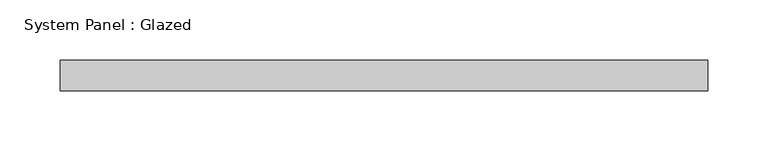
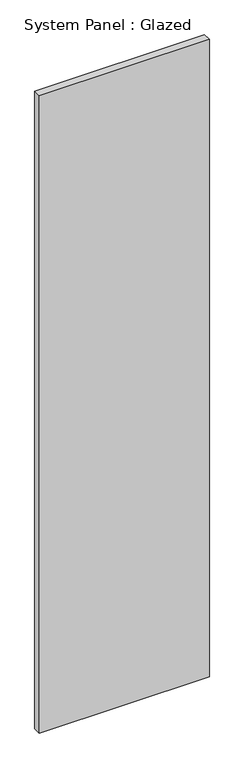
"""IFC4 building model written with IfcOpenShell, lengths in millimetres: plate geometry, System Panel : Glazed."""

from ifc_helpers import new_model, si_unit, origin, origin_with_axes, place, context, project, spatial, polyline, outline, extrude, source, transform, mapped, element, save


def system_panel_glazed_03e68811(model_context):
    return source(origin(), model_context, "Body", "SweptSolid", [
        extrude(outline(polyline([(267.5, 24.5), (-267.5, 24.5), (-267.5, 49.5), (267.5, 49.5), (267.5, 24.5)])), origin_with_axes(), (0.0, 0.0, 1.0), 2120.0),
    ])


if __name__ == "__main__":
    model = new_model("IFC4")
    model_context = context("Model", 3, world=origin())
    ifc_project = project(units=[si_unit("LENGTHUNIT", "METRE", prefix="MILLI")], contexts=[model_context])
    site = spatial("IfcSite", under=ifc_project)
    building = spatial("IfcBuilding", under=site)
    placement = place(None, origin())
    system_panel_glazed_shape = system_panel_glazed_03e68811(model_context)
    element("IfcPlate", 1, ObjectType="System Panel : Glazed", at=placement, inside=building, context=model_context, shape_type="MappedRepresentation", body=[
        mapped(system_panel_glazed_shape, transform((0.0, 0.0, 0.0), x_axis=(1.0, 0.0, 0.0), y_axis=(0.0, 1.0, 0.0), z_axis=(0.0, 0.0, 1.0))),
    ])
    save(model, "model.ifc")

# Revit data of these elements
# Type "System Panel : Glazed"
#   Construction Type Id = "GSP4R"
#   Analytic Construction = "1/8 in Pilkington single glazing"
#   Visual Light Transmittance = 0.9
#   Solar Heat Gain Coefficient = 0.86
#   Heat Transfer Coefficient (U) = 6.7069 W/(m²·K)
#   Define Thermal Properties by = 1
# Element 1 (IfcPlate, "System Panel : Glazed")
#   Materials on its faces: "Glass"
# Materials
#   "Glass": class "Glass", colour RGB 245 245 243, transparency 1, Description = "Soda Lime Glass", Cost = 0
